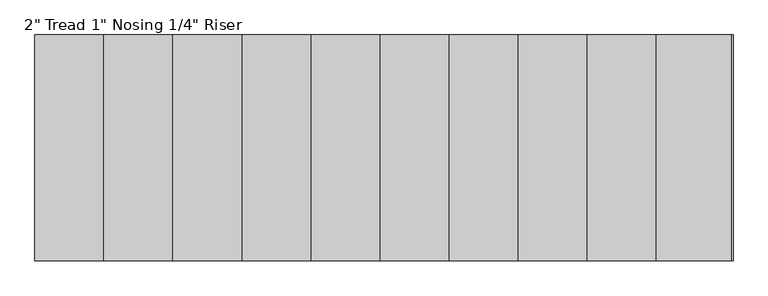
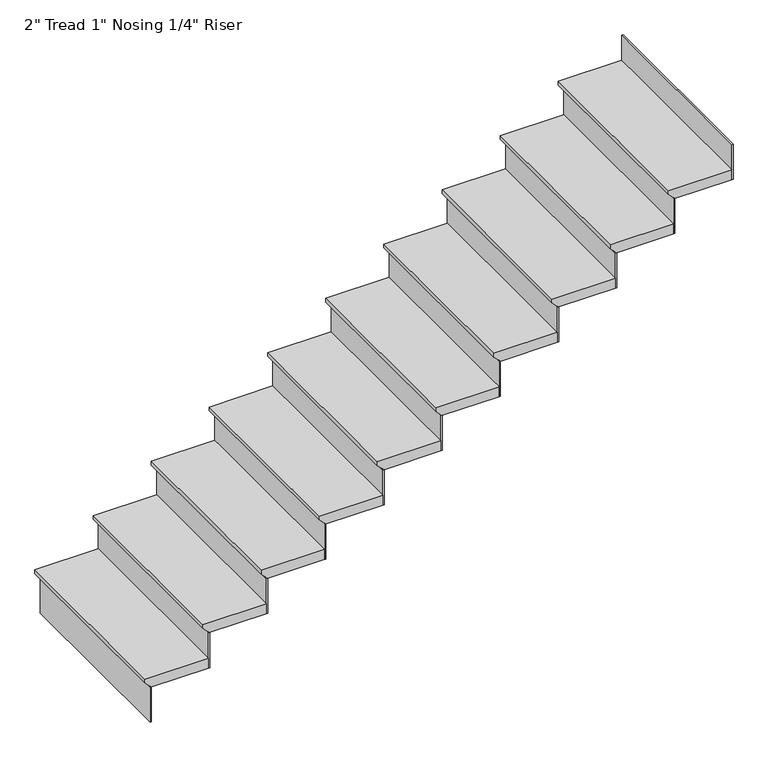
"""IFC4 building model written with IfcOpenShell, lengths in millimetres: stair flight geometry."""

from ifc_helpers import new_model, si_unit, frame, origin, place, context, project, spatial, polyline, outline, extrude, source, transform, mapped, element, save


def stair_flight_c577b9fb(model_context):
    return source(origin(), model_context, "Body", "SweptSolid", [
        extrude(outline(polyline([(5232.4, -7947.6763529), (5232.4, -8252.4763529), (5213.35, -8252.4763529), (5187.95, -8227.0763529), (5181.6, -8227.0763529), (5181.6, -7947.6763529), (5232.4, -7947.6763529)])), frame((0.0, -3490.0338022, 0.0), z_axis=(0.0, 1.0, 0.0), x_axis=(0.0, 0.0, 1.0)), (0.0, 0.0, 1.0), 914.4),
        extrude(outline(polyline([(-8220.7263529, -3490.0338022), (-8227.0763529, -3490.0338022), (-8227.0763529, -2575.6338022), (-8220.7263529, -2575.6338022), (-8220.7263529, -3490.0338022)])), frame((0.0, 0.0, 5003.8), z_axis=(0.0, 0.0, 1.0), x_axis=(1.0, 0.0, 0.0)), (0.0, 0.0, 1.0), 177.8),
        extrude(outline(polyline([(-7941.3263529, -3490.0338022), (-7947.6763529, -3490.0338022), (-7947.6763529, -2575.6338022), (-7941.3263529, -2575.6338022), (-7941.3263529, -3490.0338022)])), frame((0.0, 0.0, 5181.6), z_axis=(0.0, 0.0, 1.0), x_axis=(1.0, 0.0, 0.0)), (0.0, 0.0, 1.0), 177.8),
        extrude(outline(polyline([(5410.2, -7668.2763529), (5410.2, -7973.0763529), (5391.15, -7973.0763529), (5365.75, -7947.6763529), (5359.4, -7947.6763529), (5359.4, -7668.2763529), (5410.2, -7668.2763529)])), frame((0.0, -3490.0338022, 0.0), z_axis=(0.0, 1.0, 0.0), x_axis=(0.0, 0.0, 1.0)), (0.0, 0.0, 1.0), 914.4),
        extrude(outline(polyline([(-7661.9263529, -3490.0338022), (-7668.2763529, -3490.0338022), (-7668.2763529, -2575.6338022), (-7661.9263529, -2575.6338022), (-7661.9263529, -3490.0338022)])), frame((0.0, 0.0, 5359.4), z_axis=(0.0, 0.0, 1.0), x_axis=(1.0, 0.0, 0.0)), (0.0, 0.0, 1.0), 177.8),
        extrude(outline(polyline([(5588.0, -7388.8763529), (5588.0, -7693.6763529), (5568.95, -7693.6763529), (5543.55, -7668.2763529), (5537.2, -7668.2763529), (5537.2, -7388.8763529), (5588.0, -7388.8763529)])), frame((0.0, -3490.0338022, 0.0), z_axis=(0.0, 1.0, 0.0), x_axis=(0.0, 0.0, 1.0)), (0.0, 0.0, 1.0), 914.4),
        extrude(outline(polyline([(-7382.5263529, -3490.0338022), (-7388.8763529, -3490.0338022), (-7388.8763529, -2575.6338022), (-7382.5263529, -2575.6338022), (-7382.5263529, -3490.0338022)])), frame((0.0, 0.0, 5537.2), z_axis=(0.0, 0.0, 1.0), x_axis=(1.0, 0.0, 0.0)), (0.0, 0.0, 1.0), 177.8),
        extrude(outline(polyline([(5765.8, -7109.4763529), (5765.8, -7414.2763529), (5746.75, -7414.2763529), (5721.35, -7388.8763529), (5715.0, -7388.8763529), (5715.0, -7109.4763529), (5765.8, -7109.4763529)])), frame((0.0, -3490.0338022, 0.0), z_axis=(0.0, 1.0, 0.0), x_axis=(0.0, 0.0, 1.0)), (0.0, 0.0, 1.0), 914.4),
        extrude(outline(polyline([(-7103.1263529, -3490.0338022), (-7109.4763529, -3490.0338022), (-7109.4763529, -2575.6338022), (-7103.1263529, -2575.6338022), (-7103.1263529, -3490.0338022)])), frame((0.0, 0.0, 5715.0), z_axis=(0.0, 0.0, 1.0), x_axis=(1.0, 0.0, 0.0)), (0.0, 0.0, 1.0), 177.8),
        extrude(outline(polyline([(5943.6, -6830.0763529), (5943.6, -7134.8763529), (5924.55, -7134.8763529), (5899.15, -7109.4763529), (5892.8, -7109.4763529), (5892.8, -6830.0763529), (5943.6, -6830.0763529)])), frame((0.0, -3490.0338022, 0.0), z_axis=(0.0, 1.0, 0.0), x_axis=(0.0, 0.0, 1.0)), (0.0, 0.0, 1.0), 914.4),
        extrude(outline(polyline([(-6823.7263529, -3490.0338022), (-6830.0763529, -3490.0338022), (-6830.0763529, -2575.6338022), (-6823.7263529, -2575.6338022), (-6823.7263529, -3490.0338022)])), frame((0.0, 0.0, 5892.8), z_axis=(0.0, 0.0, 1.0), x_axis=(1.0, 0.0, 0.0)), (0.0, 0.0, 1.0), 177.8),
        extrude(outline(polyline([(6121.4, -6550.6763529), (6121.4, -6855.4763529), (6102.35, -6855.4763529), (6076.95, -6830.0763529), (6070.6, -6830.0763529), (6070.6, -6550.6763529), (6121.4, -6550.6763529)])), frame((0.0, -3490.0338022, 0.0), z_axis=(0.0, 1.0, 0.0), x_axis=(0.0, 0.0, 1.0)), (0.0, 0.0, 1.0), 914.4),
        extrude(outline(polyline([(-6544.3263529, -3490.0338022), (-6550.6763529, -3490.0338022), (-6550.6763529, -2575.6338022), (-6544.3263529, -2575.6338022), (-6544.3263529, -3490.0338022)])), frame((0.0, 0.0, 6070.6), z_axis=(0.0, 0.0, 1.0), x_axis=(1.0, 0.0, 0.0)), (0.0, 0.0, 1.0), 177.8),
        extrude(outline(polyline([(6299.2, -6271.2763529), (6299.2, -6576.0763529), (6280.15, -6576.0763529), (6254.75, -6550.6763529), (6248.4, -6550.6763529), (6248.4, -6271.2763529), (6299.2, -6271.2763529)])), frame((0.0, -3490.0338022, 0.0), z_axis=(0.0, 1.0, 0.0), x_axis=(0.0, 0.0, 1.0)), (0.0, 0.0, 1.0), 914.4),
        extrude(outline(polyline([(-6264.9263529, -3490.0338022), (-6271.2763529, -3490.0338022), (-6271.2763529, -2575.6338022), (-6264.9263529, -2575.6338022), (-6264.9263529, -3490.0338022)])), frame((0.0, 0.0, 6248.4), z_axis=(0.0, 0.0, 1.0), x_axis=(1.0, 0.0, 0.0)), (0.0, 0.0, 1.0), 177.8),
        extrude(outline(polyline([(6477.0, -5991.8763529), (6477.0, -6296.6763529), (6457.95, -6296.6763529), (6432.55, -6271.2763529), (6426.2, -6271.2763529), (6426.2, -5991.8763529), (6477.0, -5991.8763529)])), frame((0.0, -3490.0338022, 0.0), z_axis=(0.0, 1.0, 0.0), x_axis=(0.0, 0.0, 1.0)), (0.0, 0.0, 1.0), 914.4),
        extrude(outline(polyline([(-5985.5263529, -3490.0338022), (-5991.8763529, -3490.0338022), (-5991.8763529, -2575.6338022), (-5985.5263529, -2575.6338022), (-5985.5263529, -3490.0338022)])), frame((0.0, 0.0, 6426.2), z_axis=(0.0, 0.0, 1.0), x_axis=(1.0, 0.0, 0.0)), (0.0, 0.0, 1.0), 177.8),
        extrude(outline(polyline([(6654.8, -5712.4763529), (6654.8, -6017.2763529), (6635.75, -6017.2763529), (6610.35, -5991.8763529), (6604.0, -5991.8763529), (6604.0, -5712.4763529), (6654.8, -5712.4763529)])), frame((0.0, -3490.0338022, 0.0), z_axis=(0.0, 1.0, 0.0), x_axis=(0.0, 0.0, 1.0)), (0.0, 0.0, 1.0), 914.4),
        extrude(outline(polyline([(-5706.1263529, -3490.0338022), (-5712.4763529, -3490.0338022), (-5712.4763529, -2575.6338022), (-5706.1263529, -2575.6338022), (-5706.1263529, -3490.0338022)])), frame((0.0, 0.0, 6604.0), z_axis=(0.0, 0.0, 1.0), x_axis=(1.0, 0.0, 0.0)), (0.0, 0.0, 1.0), 177.8),
        extrude(outline(polyline([(-5426.7263529, -3490.0338022), (-5433.0763529, -3490.0338022), (-5433.0763529, -2575.6338022), (-5426.7263529, -2575.6338022), (-5426.7263529, -3490.0338022)])), frame((0.0, 0.0, 6781.8), z_axis=(0.0, 0.0, 1.0), x_axis=(1.0, 0.0, 0.0)), (0.0, 0.0, 1.0), 177.8),
        extrude(outline(polyline([(6832.6, -5433.0763529), (6832.6, -5737.8763529), (6813.55, -5737.8763529), (6788.15, -5712.4763529), (6781.8, -5712.4763529), (6781.8, -5433.0763529), (6832.6, -5433.0763529)])), frame((0.0, -3490.0338022, 0.0), z_axis=(0.0, 1.0, 0.0), x_axis=(0.0, 0.0, 1.0)), (0.0, 0.0, 1.0), 914.4),
    ])


if __name__ == "__main__":
    model = new_model("IFC4")
    model_context = context("Model", 3, world=origin())
    ifc_project = project(units=[si_unit("LENGTHUNIT", "METRE", prefix="MILLI")], contexts=[model_context])
    site = spatial("IfcSite", under=ifc_project)
    building = spatial("IfcBuilding", under=site)
    placement = place(None, origin())
    stair_flight_shape = stair_flight_c577b9fb(model_context)
    element("IfcStairFlight", 1, ObjectType="2\" Tread 1\" Nosing 1/4\" Riser", at=placement, inside=building, context=model_context, shape_type="MappedRepresentation", body=[
        mapped(stair_flight_shape, transform((0.0, 0.0, 0.0), x_axis=(1.0, 0.0, 0.0), y_axis=(0.0, 1.0, 0.0), z_axis=(0.0, 0.0, 1.0))),
    ])
    save(model, "model.ifc")
